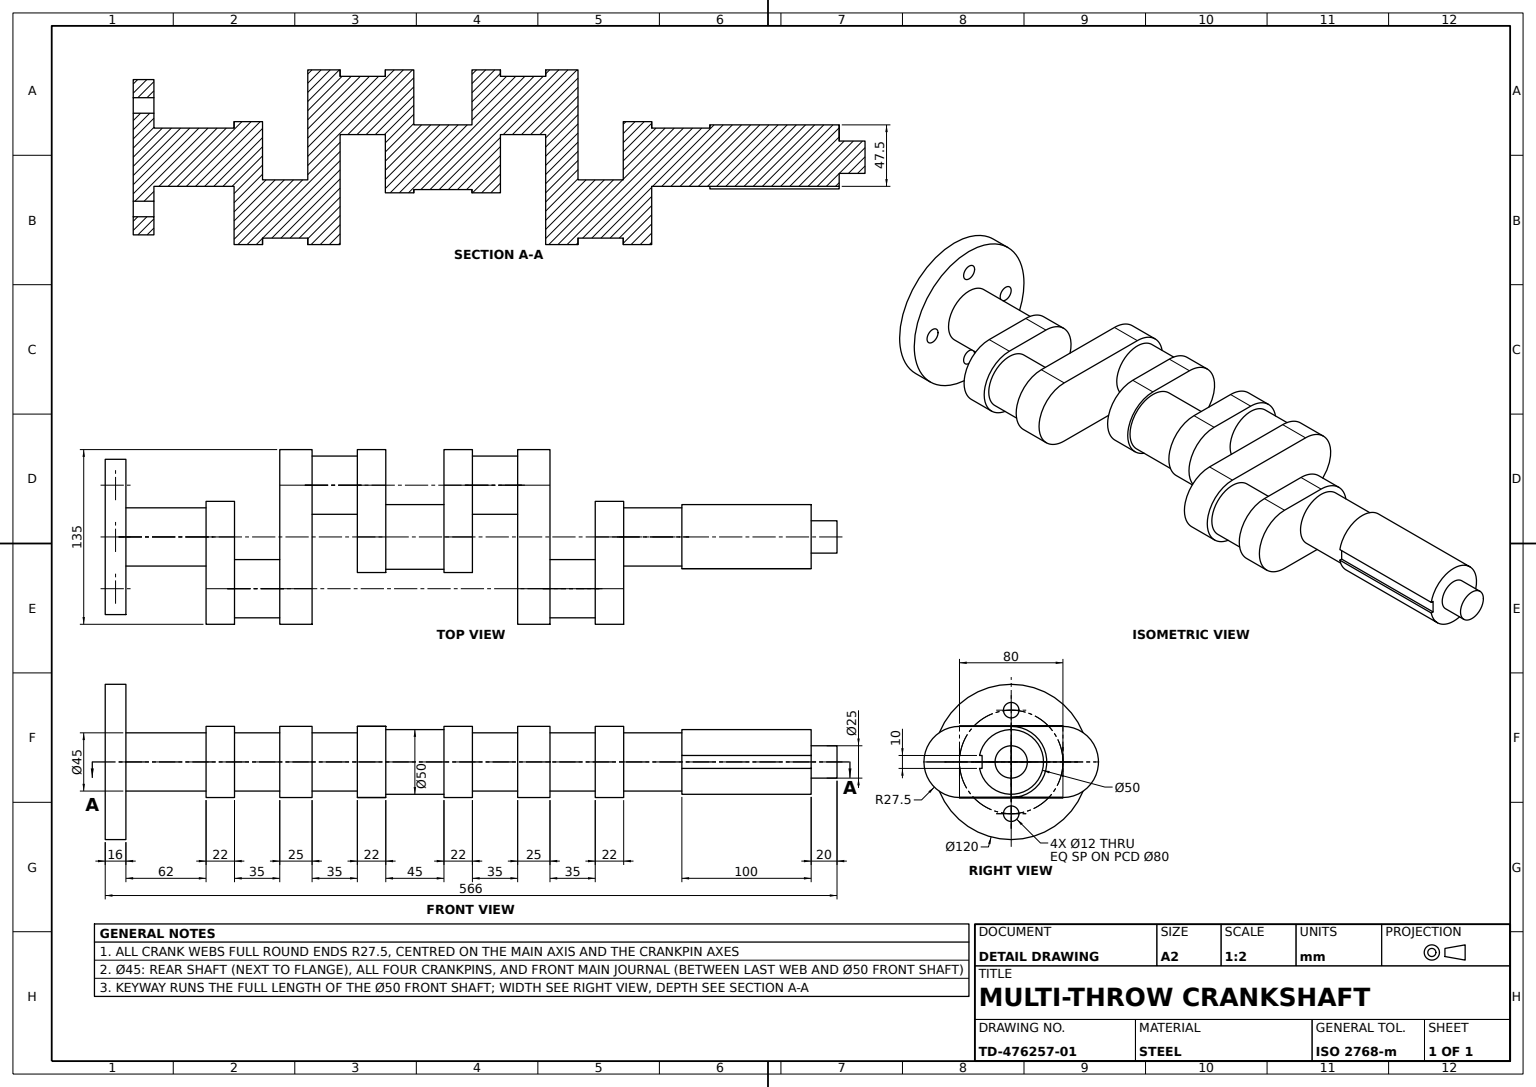
SolidWorks part; units mm, degrees
material "Plain Carbon Steel"
ref_plane "Front Plane" through (0, 0, 0) normal (0, 0, 1) x (1, 0, 0)
ref_plane "Top Plane" through (0, 0, 0) normal (0, 1, 0) x (1, 0, 0)
ref_plane "Right Plane" through (0, 0, 0) normal (1, 0, 0) x (0, 0, -1)
sketch "Flange Profile Sketch" plane through (0, 0, 0) normal (0, 0, 1) x (1, 0, 0)
  line L0 (-89.0864, 0) -> (302.0692, 0) construction
  line L1 (0, 49.5802) -> (0, -47.2099) construction
  line L2 (0, 0) -> (0, 60)
  line L3 (0, 60) -> (16, 60)
  line L4 (16, 60) -> (16, 22.5)
  line L5 (16, 22.5) -> (78, 22.5)
  line L6 (78, 22.5) -> (78, 0)
  line L7 (78, 0) -> (0, 0)
  dimension "D1" = 16
  dimension "D2" = 62
  dimension "D3" = 60
  dimension "D4" = 22.5
revolve "Flange and Rear Shaft" add sketch "Flange Profile Sketch" angle 360 about L0
sketch "Web 1 Sketch" plane through (78, 0, 0) normal (1, 0, 0) x (0, 0, -1)
  line L0 (-47.4301, 0) -> (44.8344, 0) construction
  line L1 (0, 0) -> (-40, 0) construction
  line L2 (0, -27.5) -> (-40, -27.5)
  line L3 (0, 27.5) -> (-40, 27.5)
  arc A0 (0, -27.5) -> (0, 27.5) centre (0, 0) ccw
  arc A1 (-40, 27.5) -> (-40, -27.5) centre (-40, 0) ccw
  point P5 (-20, 0)
  dimension "D1" = 27.5
  dimension "D2" = 40
extrude "Web 1" add sketch "Web 1 Sketch" along normal blind 22
sketch "Crankpin 1 Sketch" plane through (100, 0, 0) normal (1, 0, 0) x (0, 0, -1)
  circle A0 centre (-40, 0) radius 22.5
  dimension "D1" = 45
extrude "Crankpin 1 Ø45" add sketch "Crankpin 1 Sketch" along normal blind 35
sketch "Web 2 Sketch" plane through (135, 0, 0) normal (1, 0, 0) x (0, 0, -1)
  line L0 (-40, 0) -> (40, 0) construction
  line L1 (-40, 27.5) -> (40, 27.5)
  line L2 (-40, -27.5) -> (40, -27.5)
  arc A0 (-40, 27.5) -> (-40, -27.5) centre (-40, 0) ccw
  arc A1 (40, -27.5) -> (40, 27.5) centre (40, 0) ccw
  point P4 (0, 0)
  dimension "D2" = 27.5
  dimension "D1" = 80
extrude "Web 2" add sketch "Web 2 Sketch" along normal blind 25
sketch "Crankpin 2 Sketch" plane through (160, 0, 0) normal (1, 0, 0) x (0, 0, -1)
  circle A0 centre (40, 0) radius 22.5
  dimension "D1" = 45
extrude "Crankpin 2 Ø45" add sketch "Crankpin 2 Sketch" along normal blind 35
sketch "Web 3 Sketch" plane through (195, 0, 0) normal (1, 0, 0) x (0, 0, -1)
  line L0 (40, 0) -> (0, 0) construction
  line L1 (40, -27.5) -> (0, -27.5)
  line L2 (40, 27.5) -> (0, 27.5)
  arc A0 (40, -27.5) -> (40, 27.5) centre (40, 0) ccw
  arc A1 (0, 27.5) -> (0, -27.5) centre (0, 0) ccw
  point P5 (20, 0)
  dimension "D1" = 27.5
  dimension "D2" = 40
extrude "Web 3" add sketch "Web 3 Sketch" along normal blind 22
sketch "Centre Main Journal Sketch" plane through (217, 0, 0) normal (1, 0, 0) x (0, 0, -1)
  circle A0 centre (0, 0) radius 25
  dimension "D1" = 50
extrude "Centre Main Journal Ø50" add sketch "Centre Main Journal Sketch" along normal blind 45
sketch "Web 4 Sketch" plane through (262, 0, 0) normal (1, 0, 0) x (0, 0, -1)
  line L0 (0, 0) -> (40, 0) construction
  line L1 (0, 27.5) -> (40, 27.5)
  line L2 (0, -27.5) -> (40, -27.5)
  arc A0 (0, 27.5) -> (0, -27.5) centre (0, 0) ccw
  arc A1 (40, -27.5) -> (40, 27.5) centre (40, 0) ccw
  point P4 (20, 0)
  dimension "D1" = 27.5
extrude "Web 4" add sketch "Web 4 Sketch" along normal blind 22
sketch "Crankpin 3 Sketch" plane through (284, 0, 0) normal (1, 0, 0) x (0, 0, -1)
  circle A0 centre (40, 0) radius 22.5
  dimension "D1" = 45
extrude "Crankpin 3 Ø45" add sketch "Crankpin 3 Sketch" along normal blind 35
sketch "Web 5 Sketch" plane through (319, 0, 0) normal (1, 0, 0) x (0, 0, -1)
  line L0 (40, 0) -> (-40, 0) construction
  line L1 (40, -27.5) -> (-40, -27.5)
  line L2 (40, 27.5) -> (-40, 27.5)
  arc A0 (40, -27.5) -> (40, 27.5) centre (40, 0) ccw
  arc A1 (-40, 27.5) -> (-40, -27.5) centre (-40, 0) ccw
  point P4 (0, 0)
  dimension "D1" = 27.5
extrude "Web 5" add sketch "Web 5 Sketch" along normal blind 25
sketch "Crankpin 4 Sketch" plane through (344, 0, 0) normal (1, 0, 0) x (0, 0, -1)
  circle A0 centre (-40, 0) radius 22.5
  dimension "D1" = 45
extrude "Crankpin 4 Ø45" add sketch "Crankpin 4 Sketch" along normal blind 35
sketch "Web 6 Sketch" plane through (379, 0, 0) normal (1, 0, 0) x (0, 0, -1)
  line L0 (-40, 0) -> (0, 0) construction
  line L1 (-40, 27.5) -> (0, 27.5)
  line L2 (-40, -27.5) -> (0, -27.5)
  arc A0 (-40, 27.5) -> (-40, -27.5) centre (-40, 0) ccw
  arc A1 (0, -27.5) -> (0, 27.5) centre (0, 0) ccw
  point P4 (-20, 0)
  dimension "D2" = 27.5
  dimension "D1" = 40
extrude "Web 6" add sketch "Web 6 Sketch" along normal blind 22
sketch "Front Journal Sketch" plane through (401, 0, 0) normal (1, 0, 0) x (0, 0, -1)
  circle A0 centre (0, 0) radius 22.5
  dimension "D1" = 45
extrude "Front Journal Ø45" add sketch "Front Journal Sketch" along normal blind 45
sketch "Front Shaft Sketch" plane through (446, 0, 0) normal (1, 0, 0) x (0, 0, -1)
  circle A0 centre (0, 0) radius 25
  dimension "D1" = 50
extrude "Front Shaft Ø50" add sketch "Front Shaft Sketch" along normal blind 100
sketch "Nose Sketch" plane through (546, 0, 0) normal (1, 0, 0) x (0, 0, -1)
  circle A0 centre (0, 0) radius 12.5
  dimension "D1" = 25
extrude "Nose Ø25" add sketch "Nose Sketch" along normal blind 20
sketch "Flange Bolt Holes Sketch" plane through (0, 0, 0) normal (-1, 0, 0) x (0, 0, 1)
  circle A0 centre (0, 0) radius 40 construction
  circle A1 centre (0, 40) radius 6
  circle A2 centre (40, 0) radius 6
  circle A3 centre (0, -40) radius 6
  circle A4 centre (-40, 0) radius 6
  point P14 (0, 0)
  dimension "D1" = 80
  dimension "D2" = 12
  dimension "D4" = 80
  dimension "D5" = 40
  dimension "D3" = 4
extrude "Flange Bolt Holes 4xØ12" cut sketch "Flange Bolt Holes Sketch" against normal blind 20
sketch "Keyway Sketch" plane through (546, 0, 0) normal (1, 0, 0) x (0, 0, -1)
  line L0 (-49.8059, 0) -> (16.356, 0) construction
  line L2 (-27.5, 5) -> (-22.5, 5)
  line L3 (-27.5, 5) -> (-27.5, -5)
  line L4 (-27.5, -5) -> (-22.5, -5)
  line L5 (-22.5, 5) -> (-22.5, -5)
  line L6 (-27.5, 5) -> (-22.5, -5) construction
  line L7 (-27.5, -5) -> (-22.5, 5) construction
  circle A0 centre (0, 0) radius 25 construction
  point P3 (-25, 0)
  dimension "D1" = 10
  dimension "D2" = 5
extrude "Keyway 10x5" cut sketch "Keyway Sketch" against normal blind 110
